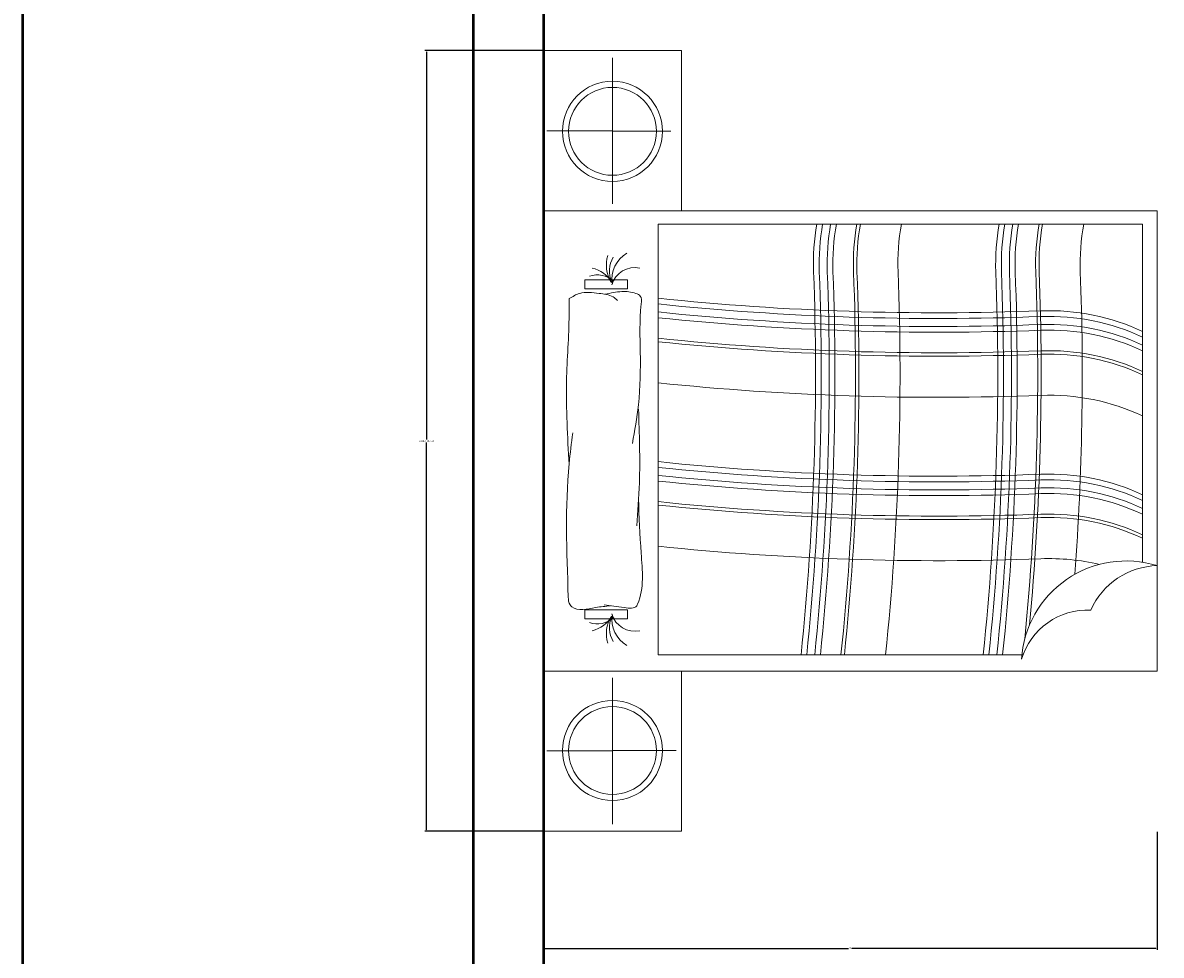
# Model space of a CAD drawing. Units: inches. Extents: x 64 to 1167, y 117 to 939.
# Tile 6 of 56: x 64 to 210, y 644 to 764. Entities that reach past the tile are written whole.
import ezdxf

# ---------------------------------------------------------------- set-up
doc = ezdxf.new("R2010")
doc.units = ezdxf.units.IN
doc.header["$MEASUREMENT"] = 0
for name, color, linetype, lineweight in [('A-ANNO-DIMS', 2, 'Continuous', 18), ('A-ANNO-TTLB', 7, 'Continuous', 50), ('A-FURN', 8, 'Continuous', 18), ('A-WALL', 7, 'Continuous', 50)]:
    doc.layers.add(name, color=color, linetype=linetype, lineweight=lineweight)
doc.styles.get("Standard").update_dxf_attribs({"font": 'arial.ttf'})
doc.dimstyles.get("Standard").update_dxf_attribs({"dimtxt": 0.18, "dimasz": 0.18, "dimexe": 0.18, "dimexo": 0.0625, "dimgap": 0.09, "dimtad": 0, "dimtih": 1, "dimtoh": 1, "dimdec": 4, "dimzin": 0, "dimdsep": 46, "dimtxsty": 'Standard', "dimcen": 0.09, "dimadec": 0, "dimazin": 0, "dimtfac": 1, "dimtdec": 4, "dimtofl": 0, "dimtmove": 0, "dimatfit": 3, "dimfxl": 1, "dimtolj": 1, "dimtzin": 0, "dimarcsym": 0})

# ---------------------------------------------------------------- blocks, each defined once
blk = doc.blocks.new('A$C55D95FC8')
for p, q in [((0.0205361354800709, 0.0787401590790205), (4.4308863e-09, 0.0787401590790205)), ((4.4308863e-09, 0.0787401590790205), (4.4308863e-09, 0.0610236236460642)), ((0.0102998515468766, 0.0698818913625423), (0.0102998515468766, 0.0782838519186531)), ((0.0795912535903072, 0.0787401590790205), (0.0205361354800709, 0.0787401590790205)), ((0.0205361354800709, 0.0787401590790205), (0.0205361354800709, 1.5987055e-09)), ((0.0205361354800709, 0.0610236236460642), (0.0205361354800709, 0.0787401590790205)), ((0.0795912535903072, 1.5987055e-09), (0.0795912535903072, 0.0787401590790205)), ((0.0795912535903072, 0.0610236236460642), (0.0795912535903072, 0.0787401590790205)), ((0.0795912535903072, 0.0787401590790205), (0.1001273846397782, 0.0787401590790205)), ((0.0898275375237879, 0.0698818913625423), (0.0898275375237879, 0.0782838519186531)), ((0.1001273846397782, 0.0787401590790205), (0.1001273846397782, 0.0610236236460642)), ((0.0272311420468307, 0.0734271749680611), (0.0272311420468307, 0.0679327835913016)), ((0.0283869636379362, 0.0734271749680611), (0.0272311420468307, 0.0734271749680611)), ((0.0283869636379362, 0.0679327835913016), (0.0283869636379362, 0.0734271749680611)), ((0.069568573495116, 0.0679327835913016), (0.069568573495116, 0.0734271749680611)), ((0.069568573495116, 0.0734271749680611), (0.0707243950862216, 0.0734271749680611)), ((0.0707243950862216, 0.0734271749680611), (0.0707243950862216, 0.0679327835913016)), ((0.0103603661252029, 0.0698818913625423), (0.0009192854205447, 0.0698818913625423)), ((0.0009192854205447, 0.0698818913625423), (0.019680417673495, 0.0698818913625423)), ((0.0103603661252029, 0.0698818913625423), (0.0103603661252029, 0.0617163444177833)), ((0.0992081036501199, 0.0698818913625423), (0.0804469713971695, 0.0698818913625423)), ((0.0897670229454617, 0.0698818913625423), (0.0897670229454617, 0.0624090651895023)), ((0.0897670229454617, 0.0698818913625423), (0.0992081036501199, 0.0698818913625423)), ((0.0272311420468307, 0.0679327835913016), (0.0283869636379362, 0.0679327835913016)), ((0.0707243950862216, 0.0679327835913016), (0.069568573495116, 0.0679327835913016)), ((0.0226420846349614, 0.017356024391621), (0.0226420846349614, 0.0640350115384886)), ((0.0226420846349614, 0.0640350115384886), (0.0778805917706643, 0.0640350115384886)), ((0.0778805917706643, 0.0640350115384886), (0.0778805917706643, 0.0018622155448969)), ((4.4308863e-09, 0.0610236236460642), (0.0205361354800709, 0.0610236236460642)), ((0.0795912535903072, 0.0610236236460642), (0.1001273846397782, 0.0610236236460642)), ((0.1001273846397782, 0.0610236236460642), (0.0795912535903072, 0.0610236236460642)), ((0.0778805917706643, 0.0018622155448969), (0.0345050036243423, 0.0018622155448969)), ((0.0205361354800709, 1.5987055e-09), (0.0795912535903072, 1.5987055e-09))]:
    blk.add_line(p, q)
for centre, radius in [((0.0103603661252029, 0.0698818913625423), 0.006419992945833), ((0.0897670229454617, 0.0698818913625423), 0.006419992945833), ((0.0103603661252029, 0.0698818913625423), 0.0056325913710299), ((0.0897670229454617, 0.0698818913625423), 0.0056325913710299)]:
    blk.add_circle(centre, radius)
for centre, radius, start, end in [((0.0296173146182802, 0.0733834517370097), 0.0039874401704988, 192.7739916162339, 239.2385972437894), ((0.0297860034947022, 0.0718366911105549), 0.0031824290151672, 161.4559187807069, 221.5545018485011), ((0.068338222514772, 0.0733834517370097), 0.0039874401704988, 300.7614027562107, 347.2260083837661), ((0.0681695336386365, 0.0718366911105549), 0.0031824290151672, 318.4454981514989, 18.54408121929302), ((0.0253608462642617, 0.0664480235661365), 0.0042190843766298, 59.21740326024974, 107.240090550001), ((0.0261646408000347, 0.0666868176479576), 0.0035934887142845, 67.83977404534224, 120.4858536700118), ((0.0725946908687905, 0.0664480235661365), 0.0042190843766298, 72.75990944999897, 120.7825967397502), ((0.0717908963330175, 0.0666868176479576), 0.0035934887142845, 59.51414632998812, 112.1602259546577), ((0.0271444530081917, 0.0660901030046154), 0.0038571282796441, 80.94857038502408, 149.487855392208), ((0.028715306796112, 0.0670206207276953), 0.0030565277454123, 106.1164156684869, 192.2669068074336), ((0.0692402303372267, 0.0670206207276953), 0.0030565277454123, 347.7330931925664, 73.88358433151303), ((0.070811084125147, 0.0660901030046154), 0.0038571282796441, 30.51214460779195, 99.05142961497592), ((0.3830432548096809, 0.0280791632984637), 0.348342304123924, 174.0753846342186, 182.1661628802728), ((0.3883180195023627, 0.0280791632984637), 0.348342304123924, 174.0753846342186, 182.1661628802728), ((0.3887575859148706, 0.0280791632984637), 0.348342304123924, 174.0753846342186, 182.1661628802728), ((0.3913949682613547, 0.0280791632984637), 0.348342304123924, 174.0753846342186, 182.1661628802728), ((0.3921275708842042, 0.0280791632984637), 0.348342304123924, 174.0753846342186, 182.1661628802728), ((0.3931532177822499, 0.0280791632984637), 0.348342304123924, 174.0753846342186, 182.1661628802728), ((0.3938858284702406, 0.0280791632984637), 0.348342304123924, 174.0753846342186, 182.1661628802728), ((0.4039957914428097, 0.0280791632984637), 0.348342304123924, 174.0753846342186, 182.1661628802728), ((0.4092705561354914, 0.0280791632984637), 0.348342304123924, 174.0753846342186, 182.1661628802728), ((0.4097101225482857, 0.0280791632984637), 0.348342304123924, 174.0753846342186, 182.1661628802728), ((0.4123475048944833, 0.0280791632984637), 0.348342304123924, 174.0753846342186, 182.1661628802728), ((0.4130801075173328, 0.0280791632984637), 0.348342304123924, 174.0753846342186, 182.1661628802728), ((0.4141057544156651, 0.0280791632984637), 0.348342304123924, 174.0753846342186, 182.1661628802728), ((0.4148383651033693, 0.0280791632984637), 0.348342304123924, 174.0753846342186, 182.1661628802728), ((0.0585979328749864, 0.3921737516037414), 0.348342304123924, 264.0753846342186, 272.1661628802729), ((0.0585979328749864, 0.3914411409160372), 0.348342304123924, 264.0753846342186, 272.1661628802729), ((0.0585979328749864, 0.3904154940179914), 0.348342304123924, 264.0753846342186, 272.1661628802729), ((0.0728352246873629, 0.015771730606617), 0.0283288812470293, 79.74090408767417, 92.16616288027289), ((0.0585979328749864, 0.3896828913948554), 0.348342304123924, 264.0753846342186, 272.1661628802729), ((0.0728352246873629, 0.0150391199189127), 0.0283288812470293, 79.74090408767417, 92.16616288027289), ((0.0728352246873629, 0.014013473020867), 0.0283288812470293, 79.74090408767417, 92.16616288027289), ((0.0728352246873629, 0.0132808703980175), 0.0283288812470293, 79.74090408767417, 92.16616288027289), ((0.0585979328749864, 0.3870455090486578), 0.348342304123924, 264.0753846342186, 272.1661628802729), ((0.0585979328749864, 0.3866059426358634), 0.348342304123924, 264.0753846342186, 272.1661628802729), ((0.0728352246873629, 0.0106434880515334), 0.0283288812470293, 79.74090408767417, 92.16616288027289), ((0.0728352246873629, 0.0102039216390255), 0.0283288812470293, 79.74090408767417, 92.16616288027289), ((0.0585979328749864, 0.3813311779431817), 0.348342304123924, 264.0753846342186, 272.1661628802729), ((0.0728352246873629, 0.0049291569463438), 0.0283288812470293, 79.74090408767417, 92.16616288027289), ((0.0585979328749864, 0.3687943406750821), 0.348342304123924, 264.0753846342186, 272.1661628802729), ((0.0585979328749864, 0.3680617299873778), 0.348342304123924, 264.0753846342186, 272.1661628802729), ((0.0585979328749864, 0.3670360830893321), 0.348342304123924, 264.0753846342186, 272.1661628802729), ((0.0728352246873629, -0.0076076803217559), 0.0283288812470293, 79.74090408767417, 92.16616288027289), ((0.0585979328749864, 0.3663034804661962), 0.348342304123924, 264.0753846342186, 272.1661628802729), ((0.0728352246873629, -0.0083402910097466), 0.0283288812470293, 79.74090408767417, 92.16616288027289), ((0.0728352246873629, -0.0093659379077923), 0.0283288812470293, 79.74090408767417, 92.16616288027289), ((0.0728352246873629, -0.0100985405306418), 0.0283288812470293, 79.74090408767417, 92.16616288027289), ((0.0195257132829971, 0.0089175451015705), 0.0088569915620492, 357.3071513036548, 73.40032815229439), ((0.0212196169191225, 0.0039785456130172), 0.0134528938473918, 342.7981496611725, 86.43553409471039), ((0.0585979328749864, 0.3636660981199986), 0.348342304123924, 264.0753846342186, 264.0894937108151), ((0.0585979328749864, 0.3636660981199986), 0.348342304123924, 264.4120534412305, 272.1661628802729), ((0.0585979328749864, 0.3632265317072041), 0.348342304123924, 264.7058345432973, 272.1661628802729), ((0.0066412338125565, 0.0138418714860871), 0.0283288812470293, 346.8653323937664, 2.166162880272892), ((0.0119159985052382, 0.0138418714860871), 0.0283288812470293, 334.9835890364534, 2.166162880272892), ((0.0123555649180327, 0.0138418714860871), 0.0283288812470293, 334.9835890364534, 2.166162880272892), ((0.0149929472642303, 0.0138418714860871), 0.0283288812470293, 334.9835890364534, 2.166162880272892), ((0.0157255498873662, 0.0138418714860871), 0.0283288812470293, 334.9835890364534, 2.166162880272892), ((0.016751196785412, 0.0138418714860871), 0.0283288812470293, 334.9835890364534, 2.166162880272892), ((0.0174838074731162, 0.0138418714860871), 0.0283288812470293, 334.9835890364534, 2.166162880272892), ((0.0275937704459717, 0.0138418714860871), 0.0283288812470293, 334.9835890364534, 2.166162880272892), ((0.0328685351386533, 0.0138418714860871), 0.0283288812470293, 334.9835890364534, 2.166162880272892), ((0.0333081015511613, 0.0138418714860871), 0.0283288812470293, 334.9835890364534, 2.166162880272892), ((0.0359454838976454, 0.0138418714860871), 0.0283288812470293, 334.9835890364534, 2.166162880272892), ((0.0366780865204949, 0.0138418714860871), 0.0283288812470293, 334.9835890364534, 2.166162880272892), ((0.0377037334185406, 0.0138418714860871), 0.0283288812470293, 334.9835890364534, 2.166162880272892), ((0.0384363441062449, 0.0138418714860871), 0.0283288812470293, 334.9835890364534, 2.166162880272892), ((0.0728352246873629, -0.0127359228771259), 0.0283288812470293, 79.74090408767417, 92.16616288027289), ((0.0728352246873629, -0.0131754892896338), 0.0283288812470293, 79.74090408767417, 92.16616288027289), ((0.0585979328749864, 0.3579517670145224), 0.348342304123924, 265.7785227093622, 272.1661628802729), ((0.0728352246873629, -0.0184502539823155), 0.0283288812470293, 79.74090408767417, 92.16616288027289), ((0.0244834742914564, -0.000265466985334), 0.0095909472211033, 1.586097126058433, 66.07543798719102)]:
    blk.add_arc(centre, radius, start, end)
for points, knots in [([(0.0289147255746749, 0.0701447881891816), (0.0288594712052914, 0.0707666941439674), (0.0287170005396645, 0.0723702479682963), (0.0281455262094743, 0.0744232961440949), (0.0291889501836656, 0.0755235765192316), (0.0357739480013107, 0.0757351649322875), (0.0427713900599432, 0.0760214157222195), (0.0497713972183686, 0.0751516000976111), (0.051088468169078, 0.0749879418518811)], [0, 0, 0, 0, 0.0019279232443725, 0.0049710549766176, 0.0052895177946404, 0.0063272755938421, 0.0234363221434042, 0.0274014956701049, 0.0274014956701049, 0.0274014956701049, 0.0274014956701049]), ([(0.0470364130787642, 0.0754384657253597), (0.0506013686523754, 0.07564578582464), (0.0570190885322222, 0.0760190085184912), (0.0641049746244027, 0.0754140398777576), (0.067634298421873, 0.0754345422204783), (0.0683097002203838, 0.0754384657253597)], [0, 0, 0, 0, 0.0106982603988616, 0.0192592690214098, 0.0212852951786921, 0.0212852951786921, 0.0212852951786921, 0.0212852951786921]), ([(0.0683097002203838, 0.0754384657253597), (0.0685785629996323, 0.0749978181994451), (0.0692883614169276, 0.0738345076164275), (0.0689879989760542, 0.0718267597932685), (0.0688314660169561, 0.0700734868061442), (0.0682477936968599, 0.0694250534881208), (0.0680845849689552, 0.0692437360376921)], [0, 0, 0, 0, 0.0015109089611112, 0.0039888034791269, 0.0058462934652882, 0.0065673037581345, 0.0065673037581345, 0.0065673037581345, 0.0065673037581345]), ([(0.0426466892757907, 0.0665405795829372), (0.0403364833463862, 0.0664591918543229), (0.0358625123679179, 0.0663015754569322), (0.0311222364787154, 0.0657829571321073), (0.0284790327939758, 0.0669409639243593), (0.0287751028145959, 0.0688563501602215), (0.028930650700047, 0.0701373888742866), (0.0290272818122281, 0.0709332093724447)], [0, 0, 0, 0, 0.0069867148814816, 0.0135305512018313, 0.0137822705123746, 0.0153750965646711, 0.0179875368665022, 0.0179875368665022, 0.0179875368665022, 0.0179875368665022]), ([(0.0688724841841856, 0.0708205784039318), (0.0690213315334265, 0.070107143775094), (0.0692949545069534, 0.0687956517965324), (0.0691851298645328, 0.0672691324631092), (0.0686504962264021, 0.0660961869497445), (0.0656526661544563, 0.0664298083427261), (0.0613786281246144, 0.0662671211550312), (0.0552270037305773, 0.0663103663654968), (0.0513776154182203, 0.0670246970487446), (0.0497377822137237, 0.0673290007662003)], [0, 0, 0, 0, 0.0021664741135038, 0.0039825841174123, 0.0046392197632741, 0.005658476376735, 0.0118501383671858, 0.0186073183783135, 0.0236221958582135, 0.0236221958582135, 0.0236221958582135, 0.0236221958582135]), ([(0.0541275087927329, 0.0665405795829372), (0.0509741201218796, 0.0664303641923825), (0.0459779361239636, 0.0662557405008272), (0.040995238978393, 0.066628395605321), (0.0391574181495652, 0.0667658459244953)], [0, 0, 0, 0, 0.009455464198777, 0.0149811025071051, 0.0149811025071051, 0.0149811025071051, 0.0149811025071051])]:
    blk.add_open_spline(points, degree=3, knots=knots)
blk = doc.blocks.new('*D76')
at = {"layer": 'A-ANNO-DIMS', "color": 0, "lineweight": -2, "transparency": 16777216}
for p, q in [((131.0447888543381, 760.0521068228113), (115.9081818230044, 760.0521068228113)), ((116.0881818230044, 759.8721068228114), (116.0881818230044, 710.1715476869874)), ((116.0881818230044, 660.1047266139192), (116.0881818230044, 709.8052857497432)), ((131.0447888543381, 659.9247266139193), (115.9081818230044, 659.9247266139193))]:
    blk.add_line(p, q, dxfattribs=at)
for points in [[(116.0581818230044, 759.8721068228114), (116.1181818230044, 759.8721068228114), (116.0881818230044, 760.0521068228113)], [(116.0581818230044, 660.1047266139192), (116.1181818230044, 660.1047266139192), (116.0881818230044, 659.9247266139193)]]:
    blk.add_solid(points, dxfattribs=at)
at = {"layer": 'Defpoints', "color": 0, "lineweight": -2, "transparency": 16777216}
for p in [(116.0881818230044, 760.0521068228113), (131.1072888543381, 760.0521068228113), (131.1072888543381, 659.9247266139193)]:
    blk.add_point(p, dxfattribs=at)
at = {"layer": 'A-ANNO-DIMS', "color": 0, "transparency": 16777216, "insert": (116.0881818230046, 709.9884167183652), "char_height": 0.18, "attachment_point": 5}
blk.add_mtext('\\A1;DOUBLE BED 100', dxfattribs=at)
blk = doc.blocks.new('*D77')
at = {"layer": 'A-ANNO-DIMS', "color": 0, "lineweight": -2, "transparency": 16777216}
for p, q in [((131.1072888543381, 659.8622266139191), (131.1072888543381, 644.7256195825854)), ((209.847446350355, 659.8622266139191), (209.847446350355, 644.7256195825854)), ((131.2872888543381, 644.9056195825852), (170.2589978888403, 644.9056195825852)), ((209.6674463503549, 644.9056195825852), (170.6957373158527, 644.9056195825852))]:
    blk.add_line(p, q, dxfattribs=at)
for points in [[(131.2872888543381, 644.9356195825853), (131.2872888543381, 644.8756195825853), (131.1072888543381, 644.9056195825852)], [(209.6674463503549, 644.9356195825853), (209.6674463503549, 644.8756195825853), (209.847446350355, 644.9056195825852)]]:
    blk.add_solid(points, dxfattribs=at)
at = {"layer": 'Defpoints', "color": 0, "lineweight": -2, "transparency": 16777216}
for p in [(131.1072888543381, 659.9247266139191), (209.847446350355, 659.9247266139191), (131.1072888543381, 644.9056195825852)]:
    blk.add_point(p, dxfattribs=at)
at = {"layer": 'A-ANNO-DIMS', "color": 0, "transparency": 16777216, "insert": (170.4773676023465, 644.9056195825852), "char_height": 0.18, "attachment_point": 5}
blk.add_mtext('\\A1;79', dxfattribs=at)

msp = doc.modelspace()

# ---------------------------------------------------------------- linework, layer by layer
at = {"layer": 'A-ANNO-TTLB'}
msp.add_lwpolyline([(64.30944150321102, 939.2206678261972), (512.7662400313202, 939.2206678261972), (512.7662400313202, 116.5466470696337), (64.30944150321102, 116.5466470696337)], close=True, dxfattribs=at)
at = {"layer": 'A-WALL'}
for p, q in [((122.1072888543381, 863.1997537567942), (122.1072888543381, 155.1997537567943)), ((131.1072888543381, 781.1997537567942), (131.1072888543381, 637.1997537567942))]:
    msp.add_line(p, q, dxfattribs=at)

# ---------------------------------------------------------------- block references
at = {"layer": 'A-FURN', "xscale": 1000, "yscale": 1000, "zscale": 1000, "rotation": 90}
msp.add_blockref('A$C55D95FC8', (209.8474479333586, 659.9247221830328), dxfattribs=at)

# ---------------------------------------------------------------- dimensions: what is measured, and where the dimension line sits
at = {"layer": 'A-ANNO-DIMS'}
dim = msp.add_linear_dim(base=(116.0881818230044, 760.0521068228113), p1=(131.1072888543381, 659.9247266139191), p2=(131.1072888543381, 760.052106822811), angle=90, text='DOUBLE BED <>', dimstyle='Standard', override={"dimdec": 0, "dimlfac": 1, "dimrnd": 0, "dimzin": 0, "dimdsep": 46, "dimlunit": 2}, dxfattribs=at)
dim.commit()
dim.dimension.update_dxf_attribs({"geometry": '*D76', "text_midpoint": (116.0881818230046, 709.9884167183652)})
dim = msp.add_linear_dim(base=(131.1072888543381, 644.9056195825852), p1=(209.847446350355, 659.9247266139191), p2=(131.1072888543381, 659.9247266139191), angle=180, dimstyle='Standard', override={"dimdec": 0, "dimlfac": 1, "dimrnd": 0, "dimzin": 0, "dimdsep": 46, "dimlunit": 2}, dxfattribs=at)
dim.commit()
dim.dimension.update_dxf_attribs({"geometry": '*D77', "text_midpoint": (170.4773676023465, 644.9056195825852)})

doc.saveas('drawing.dxf')
